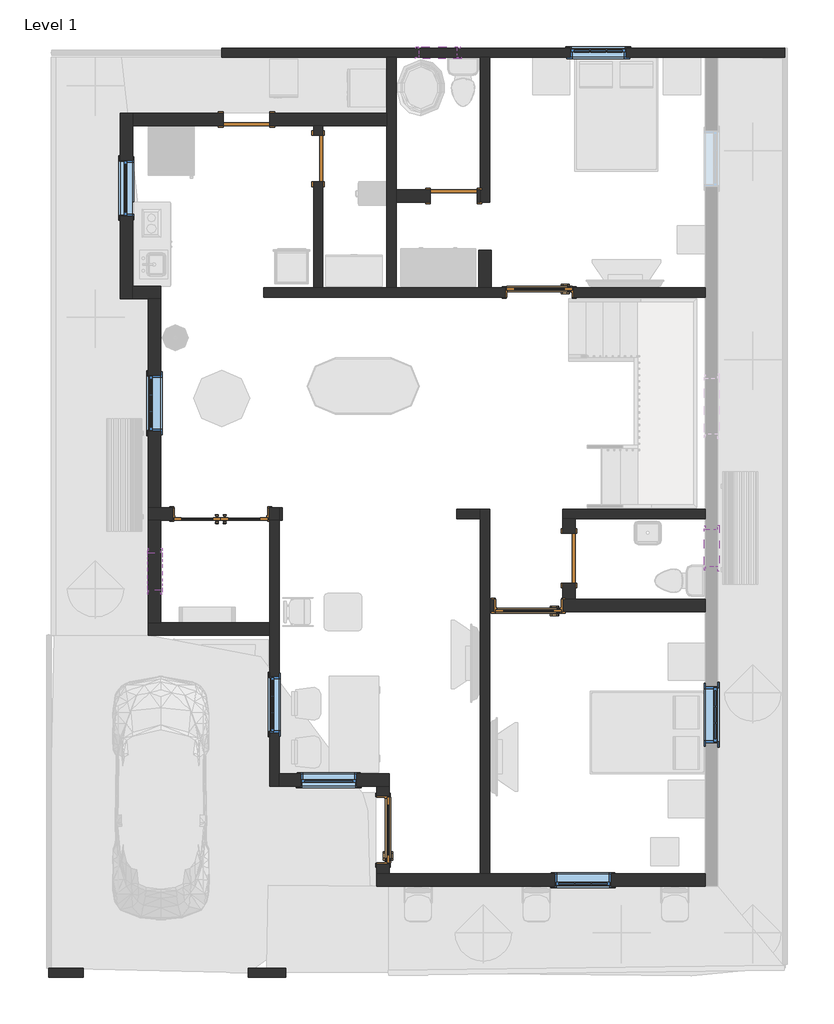
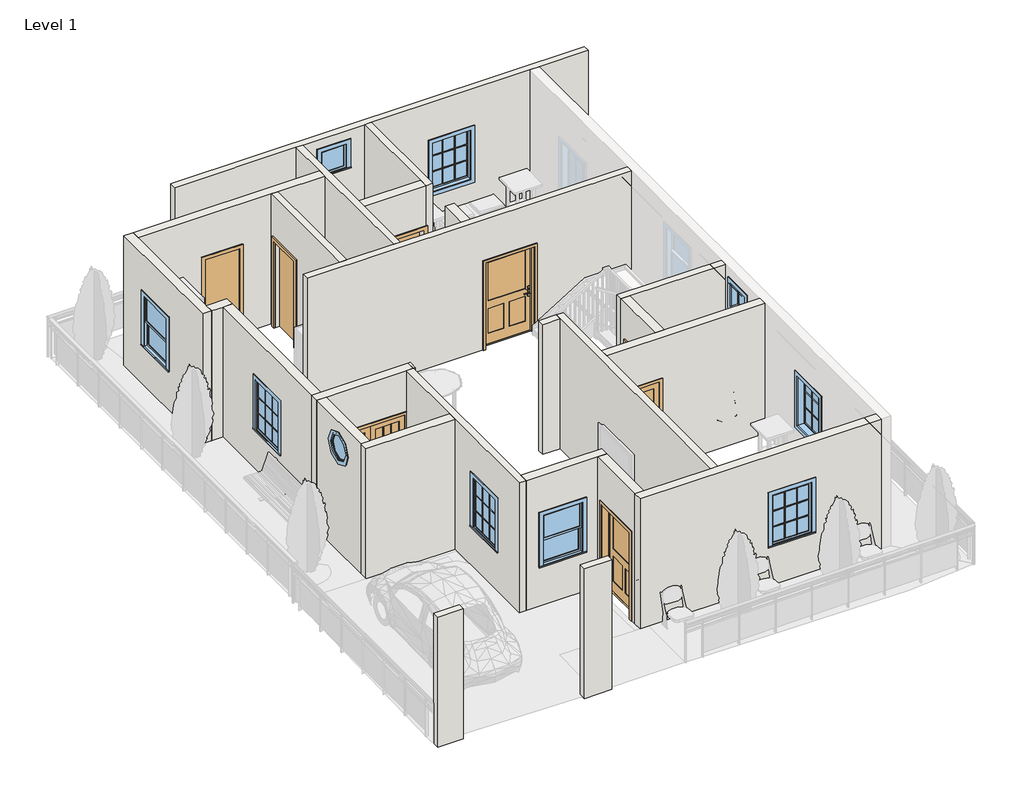
# One storey, part 1 of 4: 26 walls, 10 windows, 8 doors.
"""IFC4 building model written with IfcOpenShell, lengths in millimetres."""

from ifc_helpers import new_model, si_unit, point, frame, frame_2d, origin, origin_with_axes, place, context, project, spatial, polyline, circle_curve, trimmed, segment, composite_curve, outline, extrude, faceted_brep, transform, mapped, element, save
from components import door_e0076512, door_374e07cf, door_527a36f8, door_9d00318c, door_fadea3f2, door_53b1b562, door_255cab33, door_64d5ae29, window_bd9d39db, window_d6f340c1, window_31198920, window_3923817a, window_e41d21a6, window_3d781103

model = new_model("IFC4")

# Units and contexts
model_context = context("Model", 3, world=origin())
ifc_project = project(units=[si_unit("LENGTHUNIT", "METRE", prefix="MILLI")], contexts=[model_context])

# Site, building, storey
site = spatial("IfcSite", under=ifc_project)
building = spatial("IfcBuilding", under=site)
storey = spatial("IfcBuildingStorey", under=building, Name="Level 1", Elevation=0.0)

# Doors
placement = place(None, origin())
door_shape = door_e0076512(model_context)
element("IfcDoor", 1, ObjectType="42\" x 80\"", at=placement, inside=storey, context=model_context, shape_type="MappedRepresentation", body=[
    mapped(door_shape, transform((-11749.9684793, 2776.0018611, 0.0), x_axis=(0.0, -1.0, 0.0), y_axis=(1.0, 0.0, 0.0), z_axis=(0.0, 0.0, 1.0))),
])
door_2_shape = door_374e07cf(model_context)
element("IfcDoor", 2, ObjectType="42\" x 80\"", at=placement, inside=storey, context=model_context, shape_type="MappedRepresentation", body=[
    mapped(door_2_shape, transform((-9380.2399968, 6431.5860583, 0.0), x_axis=(1.0, 0.0, 0.0), y_axis=(0.0, 1.0, 0.0), z_axis=(0.0, 0.0, 1.0))),
])
door_3_shape = door_527a36f8(model_context)
element("IfcDoor", 3, ObjectType="42\" x 80\"", at=placement, inside=storey, context=model_context, shape_type="MappedRepresentation", body=[
    mapped(door_3_shape, transform((-9202.4399968, 11543.3360583, 0.0), x_axis=(1.0, 0.0, 0.0), y_axis=(0.0, 1.0, 0.0), z_axis=(0.0, 0.0, 1.0))),
])
door_4_shape = door_9d00318c(model_context)
element("IfcDoor", 4, ObjectType="Door-Interior-Double-Full Glass-Wood : 60\" x 80\"", at=placement, inside=storey, context=model_context, shape_type="MappedRepresentation", body=[
    mapped(door_4_shape, transform((-14396.7399968, 7927.8676639, 0.0), x_axis=(-1.0, 0.0, 0.0), y_axis=(0.0, -1.0, 0.0), z_axis=(0.0, 0.0, 1.0))),
])
door_5_shape = door_fadea3f2(model_context)
element("IfcDoor", 5, ObjectType="Single-Flush : 30\" x 80\"", at=placement, inside=storey, context=model_context, shape_type="MappedRepresentation", body=[
    mapped(door_5_shape, transform((-10599.4399968, 13114.9610583, 0.0), x_axis=(1.0, 0.0, 0.0), y_axis=(0.0, 1.0, 0.0), z_axis=(0.0, 0.0, 1.0))),
])
door_6_shape = door_53b1b562(model_context)
element("IfcDoor", 6, ObjectType="Single-Flush : 30\" x 80\"", at=placement, inside=storey, context=model_context, shape_type="MappedRepresentation", body=[
    mapped(door_6_shape, transform((-13977.6399968, 14359.5610583, 0.0), x_axis=(1.0, 0.0, 0.0), y_axis=(0.0, 1.0, 0.0), z_axis=(0.0, 0.0, 1.0))),
])
door_7_shape = door_255cab33(model_context)
element("IfcDoor", 7, ObjectType="Single-Flush : 30\" x 80\"", at=placement, inside=storey, context=model_context, shape_type="MappedRepresentation", body=[
    mapped(door_7_shape, transform((-12809.2399968, 13724.5610583, 0.0), x_axis=(0.0, 1.0, 0.0), y_axis=(-1.0, 0.0, 0.0), z_axis=(0.0, 0.0, 1.0))),
])
door_8_shape = door_64d5ae29(model_context)
element("IfcDoor", 8, ObjectType="Single-Flush : 32\" x 84\"", at=placement, inside=storey, context=model_context, shape_type="MappedRepresentation", body=[
    mapped(door_8_shape, transform((-8719.8399968, 7208.3018611, 0.0), x_axis=(0.0, -1.0, 0.0), y_axis=(1.0, 0.0, 0.0), z_axis=(0.0, 0.0, 1.0))),
])

# Walls
element("IfcWall", 9, ObjectType="Generic - 8\"", at=placement, inside=storey, context=model_context, shape_type="Brep", body=[
    faceted_brep([(-6495.3434793, 2063.6426639, 0.0), (-10015.2399968, 2063.6426639, 0.0), (-10167.6399968, 2063.6426639, 0.0), (-11651.5434793, 2063.6426639, 0.0), (-11854.7434793, 2063.6426639, 0.0), (-11854.7434793, 2063.6426639, 3048.0), (-11651.5434793, 2063.6426639, 3048.0), (-10167.6399968, 2063.6426639, 3048.0), (-10015.2399968, 2063.6426639, 3048.0), (-6495.3434793, 2063.6426639, 3048.0), (-8948.4399968, 2063.6426639, 2133.6), (-8948.4399968, 2063.6426639, 914.4), (-8034.0399968, 2063.6426639, 914.4), (-8034.0399968, 2063.6426639, 2133.6), (-6495.3434793, 1860.4426639, 0.0), (-6495.3434793, 1860.4426639, 3048.0), (-11854.7434793, 1860.4426639, 3048.0), (-11854.7434793, 1860.4426639, 0.0), (-8948.4399968, 1860.4426639, 2133.6), (-8034.0399968, 1860.4426639, 2133.6), (-8034.0399968, 1860.4426639, 914.4), (-8948.4399968, 1860.4426639, 914.4)], [[[0, 1, 2, 3, 4, 5, 6, 7, 8, 9], [10, 11, 12, 13]], [[14, 15, 16, 17], [18, 19, 20, 21]], [[4, 3, 2, 1, 0, 14, 17]], [[9, 8, 7, 6, 5, 16, 15]], [[0, 9, 15, 14]], [[5, 4, 17, 16]], [[11, 10, 18, 21]], [[12, 11, 21, 20]], [[13, 12, 20, 19]], [[10, 13, 19, 18]]]),
])
element("IfcWall", 10, ObjectType="Generic - 8\"", at=placement, inside=storey, context=model_context, shape_type="Brep", body=[
    faceted_brep([(-16035.0399968, 14461.1610583, 0.0), (-16035.0399968, 11438.5610583, 0.0), (-16035.0399968, 11438.5610583, 3048.0), (-16035.0399968, 14461.1610583, 3048.0), (-16035.0399968, 13699.1610583, 2133.6), (-16035.0399968, 12784.7610583, 2133.6), (-16035.0399968, 12784.7610583, 914.4), (-16035.0399968, 13699.1610583, 914.4), (-15831.8399968, 14461.1610583, 0.0), (-15831.8399968, 14461.1610583, 3048.0), (-15831.8399968, 14257.9610583, 3048.0), (-15831.8399968, 11641.7610583, 3048.0), (-15831.8399968, 11438.5610583, 3048.0), (-15831.8399968, 11438.5610583, 0.0), (-15831.8399968, 11641.7610583, 0.0), (-15831.8399968, 14257.9610583, 0.0), (-15831.8399968, 13699.1610583, 2133.6), (-15831.8399968, 13699.1610583, 914.4), (-15831.8399968, 12784.7610583, 914.4), (-15831.8399968, 12784.7610583, 2133.6)], [[[0, 1, 2, 3], [4, 5, 6, 7]], [[8, 9, 10, 11, 12, 13, 14, 15], [16, 17, 18, 19]], [[1, 0, 8, 15, 14, 13]], [[2, 1, 13, 12]], [[3, 2, 12, 11, 10, 9]], [[0, 3, 9, 8]], [[17, 16, 4, 7]], [[18, 17, 7, 6]], [[19, 18, 6, 5]], [[16, 19, 5, 4]]]),
])
element("IfcWall", 11, ObjectType="Generic - 8\"", at=placement, inside=storey, context=model_context, shape_type="Brep", body=[
    faceted_brep([(-13444.2399968, 3488.3610583, 0.0), (-11854.7434793, 3488.3610583, 0.0), (-11651.5434793, 3488.3610583, 0.0), (-11651.5434793, 3488.3610583, 3048.0), (-11854.7434793, 3488.3610583, 3048.0), (-13444.2399968, 3488.3610583, 3048.0), (-13093.9917381, 3488.3610583, 2133.6), (-12179.5917381, 3488.3610583, 2133.6), (-12179.5917381, 3488.3610583, 914.4), (-13093.9917381, 3488.3610583, 914.4), (-13444.2399968, 3691.5610583, 0.0), (-13444.2399968, 3691.5610583, 3048.0), (-11651.5434793, 3691.5610583, 3048.0), (-11651.5434793, 3691.5610583, 0.0), (-13093.9917381, 3691.5610583, 2133.6), (-13093.9917381, 3691.5610583, 914.4), (-12179.5917381, 3691.5610583, 914.4), (-12179.5917381, 3691.5610583, 2133.6)], [[[0, 1, 2, 3, 4, 5], [6, 7, 8, 9]], [[10, 11, 12, 13], [14, 15, 16, 17]], [[2, 1, 0, 10, 13]], [[5, 4, 3, 12, 11]], [[0, 5, 11, 10]], [[3, 2, 13, 12]], [[15, 14, 6, 9]], [[16, 15, 9, 8]], [[17, 16, 8, 7]], [[14, 17, 7, 6]]]),
])
element("IfcWall", 12, ObjectType="Generic - 8\"", at=placement, inside=storey, context=model_context, shape_type="SweptSolid", body=[
    extrude(outline(polyline([(2063.6426639, 3048.0), (3488.3610583, 3048.0), (3488.3610583, 0.0), (3334.8018611, 0.0), (3334.8018611, 2057.4), (2217.2018611, 2057.4), (2217.2018611, 0.0), (2063.6426639, 0.0), (2063.6426639, 3048.0)])), frame((-11854.7434793, 0.0, 0.0), z_axis=(1.0, 0.0, 0.0), x_axis=(0.0, 1.0, 0.0)), (0.0, 0.0, 1.0), 203.2),
])
element("IfcWall", 13, ObjectType="Generic - 8\"", at=placement, inside=storey, context=model_context, shape_type="Brep", body=[
    faceted_brep([(-13596.6399968, 14257.9610583, 2032.0), (-13596.6399968, 14257.9610583, 0.0), (-12885.4399968, 14257.9610583, 0.0), (-12733.0399968, 14257.9610583, 0.0), (-11691.6399968, 14257.9610583, 0.0), (-11691.6399968, 14257.9610583, 3048.0), (-12733.0399968, 14257.9610583, 3048.0), (-12885.4399968, 14257.9610583, 3048.0), (-15831.8399968, 14257.9610583, 3048.0), (-15831.8399968, 14257.9610583, 0.0), (-14358.6399968, 14257.9610583, 0.0), (-14358.6399968, 14257.9610583, 2032.0), (-11691.6399968, 14461.1610583, 0.0), (-13596.6399968, 14461.1610583, 0.0), (-13596.6399968, 14461.1610583, 2032.0), (-14358.6399968, 14461.1610583, 2032.0), (-14358.6399968, 14461.1610583, 0.0), (-15831.8399968, 14461.1610583, 0.0), (-15831.8399968, 14461.1610583, 3048.0), (-11691.6399968, 14461.1610583, 3048.0)], [[[0, 1, 2, 3, 4, 5, 6, 7, 8, 9, 10, 11]], [[12, 13, 14, 15, 16, 17, 18, 19]], [[10, 9, 17, 16]], [[4, 3, 2, 1, 13, 12]], [[8, 7, 6, 5, 19, 18]], [[9, 8, 18, 17]], [[5, 4, 12, 19]], [[14, 13, 1, 0]], [[15, 14, 0, 11]], [[16, 15, 11, 10]]]),
])
element("IfcWall", 14, ObjectType="Generic - 8\"", at=placement, inside=storey, context=model_context, shape_type="Brep", body=[
    faceted_brep([(-15831.8399968, 11438.5610583, 0.0), (-15577.8399968, 11438.5610583, 0.0), (-15374.6399968, 11438.5610583, 0.0), (-15374.6399968, 11438.5610583, 3048.0), (-15577.8399968, 11438.5610583, 3048.0), (-15831.8399968, 11438.5610583, 3048.0), (-15831.8399968, 11641.7610583, 0.0), (-15831.8399968, 11641.7610583, 3048.0), (-15374.6399968, 11641.7610583, 3048.0), (-15374.6399968, 11641.7610583, 0.0)], [[[0, 1, 2, 3, 4, 5]], [[6, 7, 8, 9]], [[2, 1, 0, 6, 9]], [[5, 4, 3, 8, 7]], [[0, 5, 7, 6]], [[3, 2, 9, 8]]]),
])
element("IfcWall", 15, ObjectType="Generic - 8\"", at=placement, inside=storey, context=model_context, shape_type="SweptSolid", body=[
    extrude(outline(polyline([(11438.5610583, 0.0), (8032.6426639, 0.0), (8032.6426639, 3048.0), (11438.5610583, 3048.0), (11438.5610583, 0.0)]), holes=[polyline([(10192.8018611, 2133.6), (9278.4018611, 2133.6), (9278.4018611, 914.4), (10192.8018611, 914.4), (10192.8018611, 2133.6)])]), frame((-15577.8399968, 0.0, 0.0), z_axis=(1.0, 0.0, 0.0), x_axis=(0.0, 1.0, 0.0)), (0.0, 0.0, 1.0), 203.2),
])
element("IfcWall", 16, ObjectType="Generic - 8\"", at=placement, inside=storey, context=model_context, shape_type="SweptSolid", body=[
    extrude(outline(polyline([(7829.4426639, 0.0), (6155.3610583, 0.0), (6155.3610583, 3048.0), (7829.4426639, 3048.0), (7829.4426639, 0.0)]), holes=[composite_curve([segment(trimmed(circle_curve(frame_2d((6992.4018611, 2438.4)), 304.8), [point((6687.6018611, 2438.4))], [point((7297.2018611, 2438.4))], True, "CARTESIAN"), True, "CONTINUOUS"), segment(trimmed(circle_curve(frame_2d((6992.4018611, 2438.4)), 304.8), [point((7297.2018611, 2438.4))], [point((6687.6018611, 2438.4))], True, "CARTESIAN"), True, "CONTINUOUS")], self_intersect=False)]), frame((-15577.8399968, 0.0, 0.0), z_axis=(1.0, 0.0, 0.0), x_axis=(0.0, 1.0, 0.0)), (0.0, 0.0, 1.0), 203.2),
])
element("IfcWall", 17, ObjectType="Generic - 8\"", at=placement, inside=storey, context=model_context, shape_type="Brep", body=[
    faceted_brep([(-15577.8399968, 5952.1610583, 0.0), (-13596.6399968, 5952.1610583, 0.0), (-13596.6399968, 5952.1610583, 3048.0), (-15577.8399968, 5952.1610583, 3048.0), (-15577.8399968, 6155.3610583, 0.0), (-15577.8399968, 6155.3610583, 3048.0), (-15374.6399968, 6155.3610583, 3048.0), (-13596.6399968, 6155.3610583, 3048.0), (-13596.6399968, 6155.3610583, 0.0), (-15374.6399968, 6155.3610583, 0.0)], [[[0, 1, 2, 3]], [[4, 5, 6, 7, 8, 9]], [[1, 0, 4, 9, 8]], [[3, 2, 7, 6, 5]], [[0, 3, 5, 4]], [[2, 1, 8, 7]]]),
])
element("IfcWall", 18, ObjectType="Generic - 8\"", at=placement, inside=storey, context=model_context, shape_type="Brep", body=[
    faceted_brep([(-6495.3434793, 6333.1610583, 3048.0), (-10015.2399968, 6333.1610583, 3048.0), (-10015.2399968, 6333.1610583, 0.0), (-9939.0399968, 6333.1610583, 0.0), (-9939.0399968, 6333.1610583, 2057.4), (-8821.4399968, 6333.1610583, 2057.4), (-8821.4399968, 6333.1610583, 0.0), (-6495.3434793, 6333.1610583, 0.0), (-10015.2399968, 6536.3610583, 3048.0), (-8821.4399968, 6536.3610583, 3048.0), (-8618.2399968, 6536.3610583, 3048.0), (-6495.3434793, 6536.3610583, 3048.0), (-6495.3434793, 6536.3610583, 0.0), (-8618.2399968, 6536.3610583, 0.0), (-8821.4399968, 6536.3610583, 0.0), (-8821.4399968, 6536.3610583, 2057.4), (-9939.0399968, 6536.3610583, 2057.4), (-9939.0399968, 6536.3610583, 0.0), (-10015.2399968, 6536.3610583, 0.0)], [[[0, 1, 2, 3, 4, 5, 6, 7]], [[8, 9, 10, 11, 12, 13, 14, 15, 16, 17, 18]], [[2, 18, 17, 3]], [[12, 7, 6, 14, 13]], [[1, 0, 11, 10, 9, 8]], [[0, 7, 12, 11]], [[2, 1, 8, 18]], [[5, 15, 14, 6]], [[15, 5, 4, 16]], [[16, 4, 3, 17]]]),
])
element("IfcWall", 19, ObjectType="Generic - 8\"", at=placement, inside=storey, context=model_context, shape_type="Brep", body=[
    faceted_brep([(-15577.8399968, 8032.6426639, 0.0), (-15577.8399968, 8032.6426639, 3048.0), (-15374.6399968, 8032.6426639, 3048.0), (-13444.2399968, 8032.6426639, 3048.0), (-13444.2399968, 8032.6426639, 0.0), (-13609.3399968, 8032.6426639, 0.0), (-13609.3399968, 8032.6426639, 2057.4), (-15184.1399968, 8032.6426639, 2057.4), (-15184.1399968, 8032.6426639, 0.0), (-15374.6399968, 8032.6426639, 0.0), (-15577.8399968, 7829.4426639, 3048.0), (-15577.8399968, 7829.4426639, 0.0), (-15374.6399968, 7829.4426639, 0.0), (-15184.1399968, 7829.4426639, 0.0), (-15184.1399968, 7829.4426639, 2057.4), (-13609.3399968, 7829.4426639, 2057.4), (-13609.3399968, 7829.4426639, 0.0), (-13596.6399968, 7829.4426639, 0.0), (-13444.2399968, 7829.4426639, 0.0), (-13444.2399968, 7829.4426639, 3048.0), (-13596.6399968, 7829.4426639, 3048.0), (-15374.6399968, 7829.4426639, 3048.0)], [[[0, 1, 2, 3, 4, 5, 6, 7, 8, 9]], [[10, 11, 12, 13, 14, 15, 16, 17, 18, 19, 20, 21]], [[11, 0, 9, 8, 13, 12]], [[4, 18, 17, 16, 5]], [[1, 0, 11, 10]], [[3, 2, 1, 10, 21, 20, 19]], [[4, 3, 19, 18]], [[7, 14, 13, 8]], [[14, 7, 6, 15]], [[15, 6, 5, 16]]]),
])
element("IfcWall", 20, ObjectType="Generic - 8\"", at=placement, inside=storey, context=model_context, shape_type="SweptSolid", body=[
    extrude(outline(polyline([(-13393.4399968, 7829.4426639), (-13444.2399968, 7829.4426639), (-13444.2399968, 8032.6426639), (-13393.4399968, 8032.6426639), (-13393.4399968, 7829.4426639)])), origin_with_axes(), (0.0, 0.0, 1.0), 3048.0),
])
element("IfcWall", 21, ObjectType="Generic - 8\"", at=placement, inside=storey, context=model_context, shape_type="Brep", body=[
    faceted_brep([(-8618.2399968, 6536.3610583, 0.0), (-8618.2399968, 6801.9018611, 0.0), (-8618.2399968, 6801.9018611, 2133.6), (-8618.2399968, 7614.7018611, 2133.6), (-8618.2399968, 7614.7018611, 0.0), (-8618.2399968, 7854.8426639, 0.0), (-8618.2399968, 7854.8426639, 3048.0), (-8618.2399968, 6536.3610583, 3048.0), (-8821.4399968, 6801.9018611, 2133.6), (-8821.4399968, 6801.9018611, 0.0), (-8821.4399968, 6536.3610583, 0.0), (-8821.4399968, 6536.3610583, 2057.4), (-8821.4399968, 6536.3610583, 3048.0), (-8821.4399968, 7854.8426639, 3048.0), (-8821.4399968, 7854.8426639, 0.0), (-8821.4399968, 7614.7018611, 0.0), (-8821.4399968, 7614.7018611, 2133.6)], [[[0, 1, 2, 3, 4, 5, 6, 7]], [[8, 9, 10, 11, 12, 13, 14, 15, 16]], [[15, 14, 5, 4]], [[10, 9, 1, 0]], [[7, 6, 13, 12]], [[0, 7, 12, 11, 10]], [[6, 5, 14, 13]], [[2, 1, 9, 8]], [[3, 2, 8, 16]], [[4, 3, 16, 15]]]),
])
element("IfcWall", 22, ObjectType="Generic - 8\"", at=placement, inside=storey, context=model_context, shape_type="SweptSolid", body=[
    extrude(outline(polyline([(2032.0, -10218.4399968), (0.0, -10218.4399968), (0.0, -10167.6399968), (3048.0, -10167.6399968), (3048.0, -11539.2399968), (0.0, -11539.2399968), (0.0, -10980.4399968), (2032.0, -10980.4399968), (2032.0, -10218.4399968)])), frame((0.0, 13013.3610583, 0.0), z_axis=(0.0, 1.0, 0.0), x_axis=(0.0, 0.0, 1.0)), (0.0, 0.0, 1.0), 203.2),
])
element("IfcWall", 23, ObjectType="Generic - 8\"", at=placement, inside=storey, context=model_context, shape_type="SweptSolid", body=[
    extrude(outline(polyline([(-10193.0399968, 11616.3610583), (-10193.0399968, 12225.9610583), (-9989.8399968, 12225.9610583), (-9989.8399968, 11616.3610583), (-10193.0399968, 11616.3610583)])), origin_with_axes(), (0.0, 0.0, 1.0), 3048.0),
])
element("IfcWall", 24, ObjectType="INNER WALL", at=placement, inside=storey, context=model_context, shape_type="Brep", body=[
    faceted_brep([(-13596.6399968, 7829.4426639, 0.0), (-13596.6399968, 6155.3610583, 0.0), (-13596.6399968, 5952.1610583, 0.0), (-13596.6399968, 3488.3610583, 0.0), (-13596.6399968, 3488.3610583, 3048.0), (-13596.6399968, 5952.1610583, 3048.0), (-13596.6399968, 6155.3610583, 3048.0), (-13596.6399968, 7829.4426639, 3048.0), (-13596.6399968, 5279.0610583, 2133.6), (-13596.6399968, 4364.6610583, 2133.6), (-13596.6399968, 4364.6610583, 914.4), (-13596.6399968, 5279.0610583, 914.4), (-13444.2399968, 7829.4426639, 0.0), (-13444.2399968, 7829.4426639, 3048.0), (-13444.2399968, 3691.5610583, 3048.0), (-13444.2399968, 3488.3610583, 3048.0), (-13444.2399968, 3488.3610583, 0.0), (-13444.2399968, 3691.5610583, 0.0), (-13444.2399968, 5279.0610583, 2133.6), (-13444.2399968, 5279.0610583, 914.4), (-13444.2399968, 4364.6610583, 914.4), (-13444.2399968, 4364.6610583, 2133.6)], [[[0, 1, 2, 3, 4, 5, 6, 7], [8, 9, 10, 11]], [[12, 13, 14, 15, 16, 17], [18, 19, 20, 21]], [[3, 2, 1, 0, 12, 17, 16]], [[7, 6, 5, 4, 15, 14, 13]], [[4, 3, 16, 15]], [[0, 7, 13, 12]], [[19, 18, 8, 11]], [[20, 19, 11, 10]], [[21, 20, 10, 9]], [[18, 21, 9, 8]]]),
])
element("IfcWall", 25, ObjectType="INNER WALL", at=placement, inside=storey, context=model_context, shape_type="Brep", body=[
    faceted_brep([(-11539.2399968, 11616.3610583, 0.0), (-11539.2399968, 13013.3610583, 0.0), (-11539.2399968, 13216.5610583, 0.0), (-11539.2399968, 15373.2426639, 0.0), (-11539.2399968, 15373.2426639, 3048.0), (-11539.2399968, 13216.5610583, 3048.0), (-11539.2399968, 13013.3610583, 3048.0), (-11539.2399968, 11616.3610583, 3048.0), (-11691.6399968, 11616.3610583, 0.0), (-11691.6399968, 11616.3610583, 3048.0), (-11691.6399968, 14257.9610583, 3048.0), (-11691.6399968, 14461.1610583, 3048.0), (-11691.6399968, 15373.2426639, 3048.0), (-11691.6399968, 15373.2426639, 0.0), (-11691.6399968, 14461.1610583, 0.0), (-11691.6399968, 14257.9610583, 0.0)], [[[0, 1, 2, 3, 4, 5, 6, 7]], [[8, 9, 10, 11, 12, 13, 14, 15]], [[3, 2, 1, 0, 8, 15, 14, 13]], [[7, 6, 5, 4, 12, 11, 10, 9]], [[4, 3, 13, 12]], [[0, 7, 9, 8]]]),
])
element("IfcWall", 26, ObjectType="INNER WALL", at=placement, inside=storey, context=model_context, shape_type="Brep", body=[
    faceted_brep([(-10167.6399968, 15373.2426639, 0.0), (-10167.6399968, 13216.5610583, 0.0), (-10167.6399968, 13013.3610583, 0.0), (-10167.6399968, 13013.3610583, 3048.0), (-10167.6399968, 13216.5610583, 3048.0), (-10167.6399968, 15373.2426639, 3048.0), (-10015.2399968, 15373.2426639, 0.0), (-10015.2399968, 15373.2426639, 3048.0), (-10015.2399968, 13013.3610583, 3048.0), (-10015.2399968, 13013.3610583, 0.0)], [[[0, 1, 2, 3, 4, 5]], [[6, 7, 8, 9]], [[2, 1, 0, 6, 9]], [[5, 4, 3, 8, 7]], [[0, 5, 7, 6]], [[3, 2, 9, 8]]]),
])
element("IfcWall", 27, ObjectType="INNER WALL", at=placement, inside=storey, context=model_context, shape_type="Brep", body=[
    faceted_brep([(-10015.2399968, 2063.6426639, 0.0), (-10015.2399968, 6333.1610583, 0.0), (-10015.2399968, 6536.3610583, 0.0), (-10015.2399968, 8007.2426639, 0.0), (-10015.2399968, 8007.2426639, 3048.0), (-10015.2399968, 6536.3610583, 3048.0), (-10015.2399968, 6333.1610583, 3048.0), (-10015.2399968, 2063.6426639, 3048.0), (-10167.6399968, 2063.6426639, 0.0), (-10167.6399968, 2063.6426639, 3048.0), (-10167.6399968, 7854.8426639, 3048.0), (-10167.6399968, 8007.2426639, 3048.0), (-10167.6399968, 8007.2426639, 0.0), (-10167.6399968, 7854.8426639, 0.0)], [[[0, 1, 2, 3, 4, 5, 6, 7]], [[8, 9, 10, 11, 12, 13]], [[3, 2, 1, 0, 8, 13, 12]], [[7, 6, 5, 4, 11, 10, 9]], [[0, 7, 9, 8]], [[4, 3, 12, 11]]]),
])
element("IfcWall", 28, ObjectType="INNER WALL", at=placement, inside=storey, context=model_context, shape_type="Brep", body=[
    faceted_brep([(-6495.3434793, 8007.2426639, 0.0), (-8821.4399968, 8007.2426639, 0.0), (-8821.4399968, 8007.2426639, 3048.0), (-6495.3434793, 8007.2426639, 3048.0), (-6495.3434793, 7854.8426639, 0.0), (-6495.3434793, 7854.8426639, 3048.0), (-8618.2399968, 7854.8426639, 3048.0), (-8821.4399968, 7854.8426639, 3048.0), (-8821.4399968, 7854.8426639, 0.0), (-8618.2399968, 7854.8426639, 0.0)], [[[0, 1, 2, 3]], [[4, 5, 6, 7, 8, 9]], [[1, 0, 4, 9, 8]], [[3, 2, 7, 6, 5]], [[0, 3, 5, 4]], [[2, 1, 8, 7]]]),
])
element("IfcWall", 29, ObjectType="INNER WALL", at=placement, inside=storey, context=model_context, shape_type="Brep", body=[
    faceted_brep([(-6495.3434793, 11463.9610583, 3048.0), (-13698.2399968, 11463.9610583, 3048.0), (-13698.2399968, 11463.9610583, 0.0), (-9761.2399968, 11463.9610583, 0.0), (-9761.2399968, 11463.9610583, 2057.4), (-8643.6399968, 11463.9610583, 2057.4), (-8643.6399968, 11463.9610583, 0.0), (-6495.3434793, 11463.9610583, 0.0), (-13698.2399968, 11616.3610583, 3048.0), (-12885.4399968, 11616.3610583, 3048.0), (-12733.0399968, 11616.3610583, 3048.0), (-11691.6399968, 11616.3610583, 3048.0), (-11539.2399968, 11616.3610583, 3048.0), (-10193.0399968, 11616.3610583, 3048.0), (-9989.8399968, 11616.3610583, 3048.0), (-6495.3434793, 11616.3610583, 3048.0), (-6495.3434793, 11616.3610583, 0.0), (-8643.6399968, 11616.3610583, 0.0), (-8643.6399968, 11616.3610583, 2057.4), (-9761.2399968, 11616.3610583, 2057.4), (-9761.2399968, 11616.3610583, 0.0), (-9989.8399968, 11616.3610583, 0.0), (-10193.0399968, 11616.3610583, 0.0), (-11539.2399968, 11616.3610583, 0.0), (-11691.6399968, 11616.3610583, 0.0), (-12733.0399968, 11616.3610583, 0.0), (-12885.4399968, 11616.3610583, 0.0), (-13698.2399968, 11616.3610583, 0.0)], [[[0, 1, 2, 3, 4, 5, 6, 7]], [[8, 9, 10, 11, 12, 13, 14, 15, 16, 17, 18, 19, 20, 21, 22, 23, 24, 25, 26, 27]], [[2, 27, 26, 25, 24, 23, 22, 21, 20, 3]], [[16, 7, 6, 17]], [[1, 0, 15, 14, 13, 12, 11, 10, 9, 8]], [[2, 1, 8, 27]], [[0, 7, 16, 15]], [[5, 18, 17, 6]], [[18, 5, 4, 19]], [[19, 4, 3, 20]]]),
])
element("IfcWall", 30, ObjectType="INNER WALL", at=placement, inside=storey, context=model_context, shape_type="SweptSolid", body=[
    extrude(outline(polyline([(14257.9610583, 0.0), (14105.5610583, 0.0), (14105.5610583, 2032.0), (13343.5610583, 2032.0), (13343.5610583, 0.0), (11616.3610583, 0.0), (11616.3610583, 3048.0), (14257.9610583, 3048.0), (14257.9610583, 0.0)])), frame((-12885.4399968, 0.0, 0.0), z_axis=(1.0, 0.0, 0.0), x_axis=(0.0, 1.0, 0.0)), (0.0, 0.0, 1.0), 152.4),
])
element("IfcWall", 31, ObjectType="INNER WALL", at=placement, inside=storey, context=model_context, shape_type="SweptSolid", body=[
    extrude(outline(polyline([(-10167.6399968, 7854.8426639), (-10548.6399968, 7854.8426639), (-10548.6399968, 8007.2426639), (-10167.6399968, 8007.2426639), (-10167.6399968, 7854.8426639)])), origin_with_axes(), (0.0, 0.0, 1.0), 3048.0),
])
element("IfcWall", 32, ObjectType="INNER WALL", at=placement, inside=storey, context=model_context, shape_type="SweptSolid", body=[
    extrude(outline(polyline([(-17199.9434793, 525.6426639), (-16641.1434793, 525.6426639), (-16641.1434793, 373.2426639), (-17199.9434793, 373.2426639), (-17199.9434793, 525.6426639)])), origin_with_axes(), (0.0, 0.0, 1.0), 3048.0),
])
element("IfcWall", 33, ObjectType="INNER WALL", at=placement, inside=storey, context=model_context, shape_type="SweptSolid", body=[
    extrude(outline(polyline([(-13948.7434793, 525.6426639), (-13339.1434793, 525.6426639), (-13339.1434793, 373.2426639), (-13948.7434793, 373.2426639), (-13948.7434793, 525.6426639)])), origin_with_axes(), (0.0, 0.0, 1.0), 3048.0),
])
element("IfcWall", 34, ObjectType="INNER WALL", at=placement, inside=storey, context=model_context, shape_type="Brep", body=[
    faceted_brep([(-14384.0399968, 15373.2426639, 0.0), (-11691.6399968, 15373.2426639, 0.0), (-11539.2399968, 15373.2426639, 0.0), (-10167.6399968, 15373.2426639, 0.0), (-10015.2399968, 15373.2426639, 0.0), (-6495.3434793, 15373.2426639, 0.0), (-6292.1434793, 15373.2426639, 0.0), (-5199.9434793, 15373.2426639, 0.0), (-5199.9434793, 15373.2426639, 3048.0), (-6292.1434793, 15373.2426639, 3048.0), (-6495.3434793, 15373.2426639, 3048.0), (-10015.2399968, 15373.2426639, 3048.0), (-10167.6399968, 15373.2426639, 3048.0), (-11539.2399968, 15373.2426639, 3048.0), (-11691.6399968, 15373.2426639, 3048.0), (-14384.0399968, 15373.2426639, 3048.0), (-7785.3917381, 15373.2426639, 2133.6), (-7785.3917381, 15373.2426639, 914.4), (-8699.7917381, 15373.2426639, 914.4), (-8699.7917381, 15373.2426639, 2133.6), (-11158.2399968, 15373.2426639, 2768.6), (-10548.6399968, 15373.2426639, 2768.6), (-10548.6399968, 15373.2426639, 2159.0), (-11158.2399968, 15373.2426639, 2159.0), (-14384.0399968, 15525.6426639, 0.0), (-14384.0399968, 15525.6426639, 3048.0), (-5199.9434793, 15525.6426639, 3048.0), (-5199.9434793, 15525.6426639, 0.0), (-7785.3917381, 15525.6426639, 2133.6), (-8699.7917381, 15525.6426639, 2133.6), (-8699.7917381, 15525.6426639, 914.4), (-7785.3917381, 15525.6426639, 914.4), (-11158.2399968, 15525.6426639, 2768.6), (-11158.2399968, 15525.6426639, 2159.0), (-10548.6399968, 15525.6426639, 2159.0), (-10548.6399968, 15525.6426639, 2768.6)], [[[0, 1, 2, 3, 4, 5, 6, 7, 8, 9, 10, 11, 12, 13, 14, 15], [16, 17, 18, 19], [20, 21, 22, 23]], [[24, 25, 26, 27], [28, 29, 30, 31], [32, 33, 34, 35]], [[7, 6, 5, 4, 3, 2, 1, 0, 24, 27]], [[8, 7, 27, 26]], [[15, 14, 13, 12, 11, 10, 9, 8, 26, 25]], [[0, 15, 25, 24]], [[17, 16, 28, 31]], [[18, 17, 31, 30]], [[19, 18, 30, 29]], [[16, 19, 29, 28]], [[33, 32, 20, 23]], [[34, 33, 23, 22]], [[35, 34, 22, 21]], [[32, 35, 21, 20]]]),
])

# Windows
window_shape = window_bd9d39db(model_context)
element("IfcWindow", 35, ObjectType="Casement 3x3 with Trim : 36\" x 48\"", at=placement, inside=storey, context=model_context, shape_type="MappedRepresentation", body=[
    mapped(window_shape, transform((-8491.2399968, 1962.0426639, -304.8), x_axis=(-1.0, 0.0, 0.0), y_axis=(0.0, -1.0, 0.0), z_axis=(0.0, 0.0, 1.0))),
])
element("IfcWindow", 36, ObjectType="Casement 3x3 with Trim : 36\" x 48\"", at=placement, inside=storey, context=model_context, shape_type="MappedRepresentation", body=[
    mapped(window_shape, transform((-6393.7434793, 4656.7610583, -304.8), x_axis=(0.0, -1.0, 0.0), y_axis=(1.0, 0.0, 0.0), z_axis=(0.0, 0.0, 1.0))),
])
element("IfcWindow", 37, ObjectType="Casement 3x3 with Trim : 36\" x 48\"", at=placement, inside=storey, context=model_context, shape_type="MappedRepresentation", body=[
    mapped(window_shape, transform((-15476.2399968, 9735.6018611, -304.8), x_axis=(0.0, 1.0, 0.0), y_axis=(-1.0, 0.0, 0.0), z_axis=(0.0, 0.0, 1.0))),
])
window_2_shape = window_d6f340c1(model_context)
element("IfcWindow", 38, ObjectType="Casement 3x3 with Trim : 36\" x 48\"", at=placement, inside=storey, context=model_context, shape_type="MappedRepresentation", body=[
    mapped(window_2_shape, transform((-8242.5917381, 15449.4426639, -304.8), x_axis=(1.0, 0.0, 0.0), y_axis=(0.0, 1.0, 0.0), z_axis=(0.0, 0.0, 1.0))),
])
element("IfcWindow", 39, ObjectType="Casement 3x3 with Trim : 36\" x 48\"", at=placement, inside=storey, context=model_context, shape_type="MappedRepresentation", body=[
    mapped(window_2_shape, transform((-13520.4399968, 4821.8610583, -304.8), x_axis=(0.0, 1.0, 0.0), y_axis=(-1.0, 0.0, 0.0), z_axis=(0.0, 0.0, 1.0))),
])
window_3_shape = window_31198920(model_context)
element("IfcWindow", 40, ObjectType="Double Hung with Trim : 36\" x 48\"", at=placement, inside=storey, context=model_context, shape_type="MappedRepresentation", body=[
    mapped(window_3_shape, transform((-15933.4399968, 13241.9610583, 0.0), x_axis=(0.0, 1.0, 0.0), y_axis=(-1.0, 0.0, 0.0), z_axis=(0.0, 0.0, 1.0))),
])
element("IfcWindow", 41, ObjectType="Double Hung with Trim : 36\" x 48\"", at=placement, inside=storey, context=model_context, shape_type="MappedRepresentation", body=[
    mapped(window_3_shape, transform((-12636.7917381, 3589.9610583, 0.0), x_axis=(-1.0, 0.0, 0.0), y_axis=(0.0, -1.0, 0.0), z_axis=(0.0, 0.0, 1.0))),
])
window_4_shape = window_3923817a(model_context)
element("IfcWindow", 42, ObjectType="Round with Trim : 48\" Diameter", at=placement, inside=storey, context=model_context, shape_type="MappedRepresentation", body=[
    mapped(window_4_shape, transform((-15476.2399968, 7144.8018611, 1524.0), x_axis=(0.0, 1.0, 0.0), y_axis=(-1.0, 0.0, 0.0), z_axis=(0.0, 0.0, 1.0))),
])
window_5_shape = window_e41d21a6(model_context)
element("IfcWindow", 43, ObjectType="Transom with Trim : 24\" x 24\"", at=placement, inside=storey, context=model_context, shape_type="MappedRepresentation", body=[
    mapped(window_5_shape, transform((-6393.7434793, 7334.1426639, 0.0), x_axis=(0.0, -1.0, 0.0), y_axis=(1.0, 0.0, 0.0), z_axis=(0.0, 0.0, 1.0))),
])
window_6_shape = window_3d781103(model_context)
element("IfcWindow", 44, ObjectType="Transom with Trim : 24\" x 24\"", at=placement, inside=storey, context=model_context, shape_type="MappedRepresentation", body=[
    mapped(window_6_shape, transform((-10891.5399968, 15449.4426639, 0.0), x_axis=(-1.0, 0.0, 0.0), y_axis=(0.0, -1.0, 0.0), z_axis=(0.0, 0.0, 1.0))),
])

save(model, "model.ifc")

# Revit data of these elements
# Type "42\" x 80\""
#   Type Mark = "8"
#   Assembly Code = "B2030100"
#   Analytic Construction = "French door, wood frame with single glass"
#   Top Rail = 0' - 4 3/4"
#   Threshold Offset [instance default] = 0' - 0 1/2"
#   Thickness = 0' - 1 3/8"
#   Thermal Resistance (R) = 1.0696 (h·ft²·°F)/BTU
#   Swing Angle [instance default] = 90.00°
#   Stiles = 0' - 4 3/4"
#   Rough Width = 3' - 8"
#   Rough Height = 6' - 9"
#   Lock Rail = 0' - 7 1/8"
#   Height = 6' - 8"
#   Width = 3' - 6"
#   Heat Transfer Coefficient (U) = 0.9350 BTU/(h·ft²·°F)
#   Door Offset [instance default] = 0' - 0"
#   Bottom Rail = 0' - 9 1/2"
#   Threshold [instance default] = yes
#   Function = 1
#   Exterior Trim [instance default] = yes
#   Trim Material = Cherry
#   Threshold Material = Cherry
#   Panel Material = Cherry
#   Glazing = Glass
#   Frame Material = Cherry
#   Door Handle Material = Aluminum
#   Visual Light Transmittance = 0
#   Solar Heat Gain Coefficient = 0
#   Wall Closure = (empty or 0)
#   Construction Type = (empty or 0)
# Type "Door-Interior-Double-Full Glass-Wood : 60\" x 80\""
#   Type Mark = "9"
#   Assembly Code = "C1020300"
#   Analytic Construction = "French door, wood frame with single glass"
#   Top Rail = 0' - 4 11/16"
#   Thickness = 0' - 1 3/8"
#   Thermal Resistance (R) = 1.0696 (h·ft²·°F)/BTU
#   Swing Angle [instance default] = 90.00°
#   Stiles = 0' - 4 3/4"
#   Rough Width = 5' - 2"
#   Rough Height = 6' - 9"
#   Panel Width = 2' - 6"
#   Height = 6' - 8"
#   Width = 5' - 0"
#   Heat Transfer Coefficient (U) = 0.9350 BTU/(h·ft²·°F)
#   Bottom Rail = 0' - 9 1/8"
#   Show Grill [instance default] = yes
#   Trim Material = Cherry
#   Panel Material = Cherry
#   Frame Material = Cherry
#   Door Handle Material = Aluminum
#   Visual Light Transmittance = 0
#   Solar Heat Gain Coefficient = 0
#   Wall Closure = (empty or 0)
#   Function = (empty or 0)
# Type "Single-Flush : 30\" x 80\""
#   Type Mark = "5"
#   Construction Type Id = "MDOOR"
#   Assembly Code = "C1020"
#   Analytic Construction = "Metal"
#   Thickness = 0' - 2"
#   Heat Transfer Coefficient (U) = 0.651978 BTU/(h·ft²·°F)
#   Height = 6' - 8"
#   Trim Projection Ext = 0' - 1"
#   Trim Projection Int = 0' - 1"
#   Trim Width = 0' - 3"
#   Width = 2' - 6"
#   Define Thermal Properties by = 1
#   Door Material = Door - Panel
#   Frame Material = Door - Frame
#   Visual Light Transmittance = 0
#   Solar Heat Gain Coefficient = 0
#   Function = (empty or 0)
#   Wall Closure = (empty or 0)
# Type "Single-Flush : 32\" x 84\""
#   Type Mark = "3"
#   Construction Type Id = "MDOOR"
#   Assembly Code = "C1020"
#   Analytic Construction = "Metal"
#   Thickness = 0' - 2"
#   Heat Transfer Coefficient (U) = 0.651978 BTU/(h·ft²·°F)
#   Height = 7' - 0"
#   Trim Projection Ext = 0' - 1"
#   Trim Projection Int = 0' - 1"
#   Trim Width = 0' - 3"
#   Width = 2' - 8"
#   Define Thermal Properties by = 1
#   Door Material = Door - Panel
#   Frame Material = Door - Frame
#   Visual Light Transmittance = 0
#   Solar Heat Gain Coefficient = 0
#   Function = (empty or 0)
#   Wall Closure = (empty or 0)
# Type "Generic - 8\""
#   Assembly Code = "B2010"
#   Layers, outside or top first: 0' - 8" "Brick, Common" (function 1)
# Type "INNER WALL"
#   Assembly Code = "B2010"
#   Layers, outside or top first: 0' - 6" "Brick, Soldier Course" (function 1)
# Type "Casement 3x3 with Trim : 36\" x 48\""
#   Type Mark = "10"
#   Construction Type Id = "GSP4R"
#   Assembly Code = "B2020100"
#   Analytic Construction = "1/8 in Pilkington single glazing"
#   Visual Light Transmittance = 0.9
#   Solar Heat Gain Coefficient = 0.78
#   Heat Transfer Coefficient (U) = 0.6496 BTU/(h·ft²·°F)
#   Height = 4' - 0"
#   Default Sill Height = 4' - 0"
#   Trim Projection - Ext. = 0' - 0 1/2"
#   Trim Projection - Int. = 0' - 0 3/4"
#   Trim Width - Exterior = 0' - 3 1/2"
#   Trim Width - Interior = 0' - 3 1/2"
#   Width = 3' - 0"
#   Window Inset = 0' - 0 3/4"
#   Define Thermal Properties by = 1
#   Glass Pane Material = Glass
#   Sash Material = Sash
#   Trim Exterior Material = Trim
#   Trim Interior Material = Trim
#   Wall Closure = (empty or 0)
# Type "Double Hung with Trim : 36\" x 48\""
#   Type Mark = "13"
#   Construction Type Id = "GSP4R"
#   Assembly Code = "B2020100"
#   Analytic Construction = "1/8 in Pilkington single glazing"
#   Visual Light Transmittance = 0.9
#   Solar Heat Gain Coefficient = 0.78
#   Heat Transfer Coefficient (U) = 0.6496 BTU/(h·ft²·°F)
#   Height = 4' - 0"
#   Default Sill Height = 3' - 0"
#   Trim Projection - Ext. = 0' - 0 1/2"
#   Trim Projection - Int. = 0' - 0 3/4"
#   Trim Width - Exterior = 0' - 3 1/2"
#   Trim Width - Interior = 0' - 3 1/2"
#   Width = 3' - 0"
#   Window Inset = 0' - 0 3/4"
#   Define Thermal Properties by = 1
#   Glass Pane Material = Glass
#   Sash Material = Sash
#   Trim Exterior Material = Trim
#   Trim Interior Material = Trim
#   Wall Closure = (empty or 0)
# Type "Round with Trim : 48\" Diameter"
#   Type Mark = "32"
#   Construction Type Id = "GSP4R"
#   Assembly Code = "B2020100"
#   Analytic Construction = "1/8 in Pilkington single glazing"
#   Visual Light Transmittance = 0.9
#   Solar Heat Gain Coefficient = 0.78
#   Heat Transfer Coefficient (U) = 0.6496 BTU/(h·ft²·°F)
#   Default Sill Height = 2' - 0"
#   Trim Projection - Ext. = 0' - 0 1/2"
#   Trim Projection - Int. = 0' - 0 3/4"
#   Trim Width - Exterior = 0' - 3 1/2"
#   Trim Width - Interior = 0' - 3 1/2"
#   Width = 2' - 0"
#   Define Thermal Properties by = 1
#   Glass Pane Material = Glass
#   Sash Material = Sash
#   Trim Exterior Material = Trim
#   Trim Interior Material = Trim
#   Wall Closure = (empty or 0)
# Type "Transom with Trim : 24\" x 24\""
#   Type Mark = "22"
#   Construction Type Id = "GSP4R"
#   Assembly Code = "B2020100"
#   Analytic Construction = "1/8 in Pilkington single glazing"
#   Visual Light Transmittance = 0.9
#   Solar Heat Gain Coefficient = 0.78
#   Heat Transfer Coefficient (U) = 0.6496 BTU/(h·ft²·°F)
#   Height = 2' - 0"
#   Default Sill Height = 7' - 1"
#   Trim Projection - Ext. = 0' - 0 1/2"
#   Trim Projection - Int. = 0' - 0 3/4"
#   Trim Width - Exterior = 0' - 3 1/2"
#   Trim Width - Interior = 0' - 3 1/2"
#   Width = 2' - 0"
#   Window Inset = 0' - 0 3/4"
#   Define Thermal Properties by = 1
#   Glass Pane Material = Glass
#   Sash Material = Sash
#   Trim Exterior Material = Trim
#   Trim Interior Material = Trim
#   Wall Closure = (empty or 0)
# Elements 1, 2, 3 (IfcDoor, "42\" x 80\"")
#   Threshold Offset = 0' - 0 1/2"
#   Swing Angle = 90.00°
#   Door Offset = 0' - 0"
#   Threshold = yes
#   Exterior Trim = yes
#   Phase Created = New Construction
#   Materials on its faces: "Cherry", "Aluminum", "Glass"
# Element 4 (IfcDoor, "Door-Interior-Double-Full Glass-Wood : 60\" x 80\"")
#   Swing Angle = 90.00°
#   Show Grill = yes
#   Phase Created = New Construction
#   Materials on its faces: "Cherry", "Aluminum", "Glass"
# Elements 5, 6, 7 (IfcDoor, "Single-Flush : 30\" x 80\"")
#   Phase Created = New Construction
#   Materials on its faces: "Door - Frame", "Door - Panel"
# Element 8 (IfcDoor, "Single-Flush : 32\" x 84\"")
#   Phase Created = New Construction
#   Materials on its faces: "Door - Frame", "Door - Panel"
# Elements 9, 10, 11, 12, 13, 14, 15, 16, 17, 18, 20, 21, 22, 23 (IfcWall, "Generic - 8\"")
#   Top Offset = 0' - 0"
#   Base Offset = 0' - 0"
#   Unconnected Height = 10' - 0"
#   wall height = 10' - 0"
#   Phase Created = New Construction
#   Base Constraint = Level 1
#   Materials on its faces: "Brick, Common"
# Element 19 (IfcWall, "Generic - 8\"")
#   Top Offset = 0' - 0"
#   Base Offset = 0' - 0"
#   Unconnected Height = 10' - 0"
#   wall height = 10' - 0"
#   Phase Created = New Construction
#   Base Constraint = Level 1
#   Materials on its faces: "Brick, Common", "Brick, Soldier Course"
# Elements 24, 26, 28 (IfcWall, "INNER WALL")
#   Top Offset = 0' - 0"
#   Base Offset = 0' - 0"
#   Unconnected Height = 10' - 0"
#   wall height = 10' - 0"
#   Phase Created = New Construction
#   Base Constraint = Level 1
#   Materials on its faces: "Brick, Soldier Course", "Brick, Common"
# Elements 25, 27, 29, 30, 31, 32, 33, 34 (IfcWall, "INNER WALL")
#   Top Offset = 0' - 0"
#   Base Offset = 0' - 0"
#   Unconnected Height = 10' - 0"
#   wall height = 10' - 0"
#   Phase Created = New Construction
#   Base Constraint = Level 1
#   Materials on its faces: "Brick, Soldier Course"
# Element 35 (IfcWindow, "Casement 3x3 with Trim : 36\" x 48\"")
#   Mark = "1"
#   Phase Created = New Construction
#   Materials on its faces: "Sash", "Glass", "Trim"
# Element 36 (IfcWindow, "Casement 3x3 with Trim : 36\" x 48\"")
#   Mark = "2"
#   Phase Created = New Construction
#   Materials on its faces: "Sash", "Glass", "Trim"
# Element 37 (IfcWindow, "Casement 3x3 with Trim : 36\" x 48\"")
#   Mark = "6"
#   Phase Created = New Construction
#   Materials on its faces: "Sash", "Glass", "Trim"
# Element 38 (IfcWindow, "Casement 3x3 with Trim : 36\" x 48\"")
#   Mark = "5"
#   Phase Created = New Construction
#   Materials on its faces: "Sash", "Glass", "Trim"
# Element 39 (IfcWindow, "Casement 3x3 with Trim : 36\" x 48\"")
#   Mark = "7"
#   Phase Created = New Construction
#   Materials on its faces: "Sash", "Glass", "Trim"
# Element 40 (IfcWindow, "Double Hung with Trim : 36\" x 48\"")
#   Mark = "8"
#   Phase Created = New Construction
#   Materials on its faces: "Sash", "Trim", "Glass"
# Element 41 (IfcWindow, "Double Hung with Trim : 36\" x 48\"")
#   Mark = "9"
#   Phase Created = New Construction
#   Materials on its faces: "Sash", "Trim", "Glass"
# Element 42 (IfcWindow, "Round with Trim : 48\" Diameter")
#   Mark = "13"
#   Phase Created = New Construction
#   Materials on its faces: "Trim", "Sash", "Glass"
# Element 43 (IfcWindow, "Transom with Trim : 24\" x 24\"")
#   Mark = "11"
#   Phase Created = New Construction
#   Materials on its faces: "Sash", "Trim", "Glass"
# Element 44 (IfcWindow, "Transom with Trim : 24\" x 24\"")
#   Mark = "12"
#   Phase Created = New Construction
#   Materials on its faces: "Sash", "Trim", "Glass"
# Materials
#   "Cherry": class "Wood", colour RGB 226 177 128, transparency 0, Description = "Prunus Serotina", Cost = 0
#   "Glass": class "Glass", colour RGB 0 128 192, transparency 0.75, Description = "Soda Lime Glass", Cost = 0
#   "Aluminum": class "Metal", colour RGB 247 247 247, transparency 0, Description = "Aluminum 6061", Cost = 0
#   "Door - Panel": class "Wood", colour RGB 210 159 95, transparency 0
#   "Door - Frame": colour RGB 118 70 51, transparency 0
#   "Brick, Common": class "Masonry", colour RGB 170 98 104, transparency 0, Description = "Common brick", Cost = 0
#   "Brick, Soldier Course": class "Masonry", colour RGB 170 98 104, transparency 0, Description = "Common brick soldier coursed", Cost = 0
#   "Sash": class "Wood", colour RGB 224 178 126, transparency 0
#   "Trim": class "Wood", colour RGB 224 178 126, transparency 0
# Room at (-15415.113, 3667.009) mm, phase "New Construction", upper level "Level 1", upper offset 10' - 0", lower offset 0' - 0"
#   Number = "1"
#   Name = "PARKING"
# Room at (-12778.773, 2404.853) mm, phase "New Construction", upper level "Level 1", upper offset 10' - 0", lower offset 0' - 0"
#   Number = "2"
#   Name = "Landing"
# Room at (-8921.392, 1142.698) mm, phase "New Construction", upper level "Level 1", upper offset 10' - 0", lower offset 0' - 0"
#   Number = "3"
#   Name = "GARDEN"
# Room at (-8172.116, 13796.104) mm, phase "New Construction", upper level "Level 1", upper offset 10' - 0", lower offset 0' - 0"
#   Number = "4"
#   Name = "BED ROOM"
# Room at (-7700.35, 9938.722) mm, phase "New Construction", upper level "Level 1", upper offset 10' - 0", lower offset 0' - 0"
#   Number = "5"
#   Name = "STAIR"
# Room at (-7700.35, 7330.133) mm, phase "New Construction", upper level "Level 1", upper offset 10' - 0", lower offset 0' - 0"
#   Number = "6"
# Room at (-8172.116, 4360.782) mm, phase "New Construction", upper level "Level 1", upper offset 10' - 0", lower offset 0' - 0"
#   Number = "7"
#   Name = "BED ROOM"
# Room at (-10949.973, 2404.853) mm, phase "New Construction", upper level "Level 1", upper offset 10' - 0", lower offset 0' - 0"
#   Number = "8"
#   Name = "Foyer"
# Room at (-11668.735, 6067.978) mm, phase "New Construction", upper level "Level 1", upper offset 10' - 0", lower offset 0' - 0"
#   Number = "9"
#   Name = "DRAWING"
# Room at (-14607.573, 6442.103) mm, phase "New Construction", upper level "Level 1", upper offset 10' - 0", lower offset 0' - 0"
#   Number = "10"
#   Name = "PRAYER"
# Room at (-16441.898, 10937.756) mm, phase "New Construction", upper level "Level 1", upper offset 10' - 0", lower offset 0' - 0"
#   Number = "11"
#   Name = "GARDEN"
# Room at (-12778.773, 14628.632) mm, phase "New Construction", upper level "Level 1", upper offset 10' - 0", lower offset 0' - 0"
#   Number = "12"
#   Name = "Utility"
# Room at (-10750.192, 14628.632) mm, phase "New Construction", upper level "Level 1", upper offset 10' - 0", lower offset 0' - 0"
#   Number = "13"
# Room at (-12057.248, 12766.556) mm, phase "New Construction", upper level "Level 1", upper offset 10' - 0", lower offset 0' - 0"
#   Number = "14"
#   Name = "STORE"
# Room at (-10851.792, 12170.806) mm, phase "New Construction", upper level "Level 1", upper offset 10' - 0", lower offset 0' - 0"
#   Number = "15"
#   Name = "Dresser"
# Room at (-14196.732, 12840.964) mm, phase "New Construction", upper level "Level 1", upper offset 10' - 0", lower offset 0' - 0"
#   Number = "16"
#   Name = "KITCHEN"
# Room at (-11668.735, 9032.958) mm, phase "New Construction", upper level "Level 1", upper offset 10' - 0", lower offset 0' - 0"
#   Number = "17"
# Room at (-5580.1, 8216.493) mm, phase "New Construction", upper level "Level 1", upper offset 10' - 0", lower offset 0' - 0"
#   Number = "18"
#   Name = "GARDEN"
